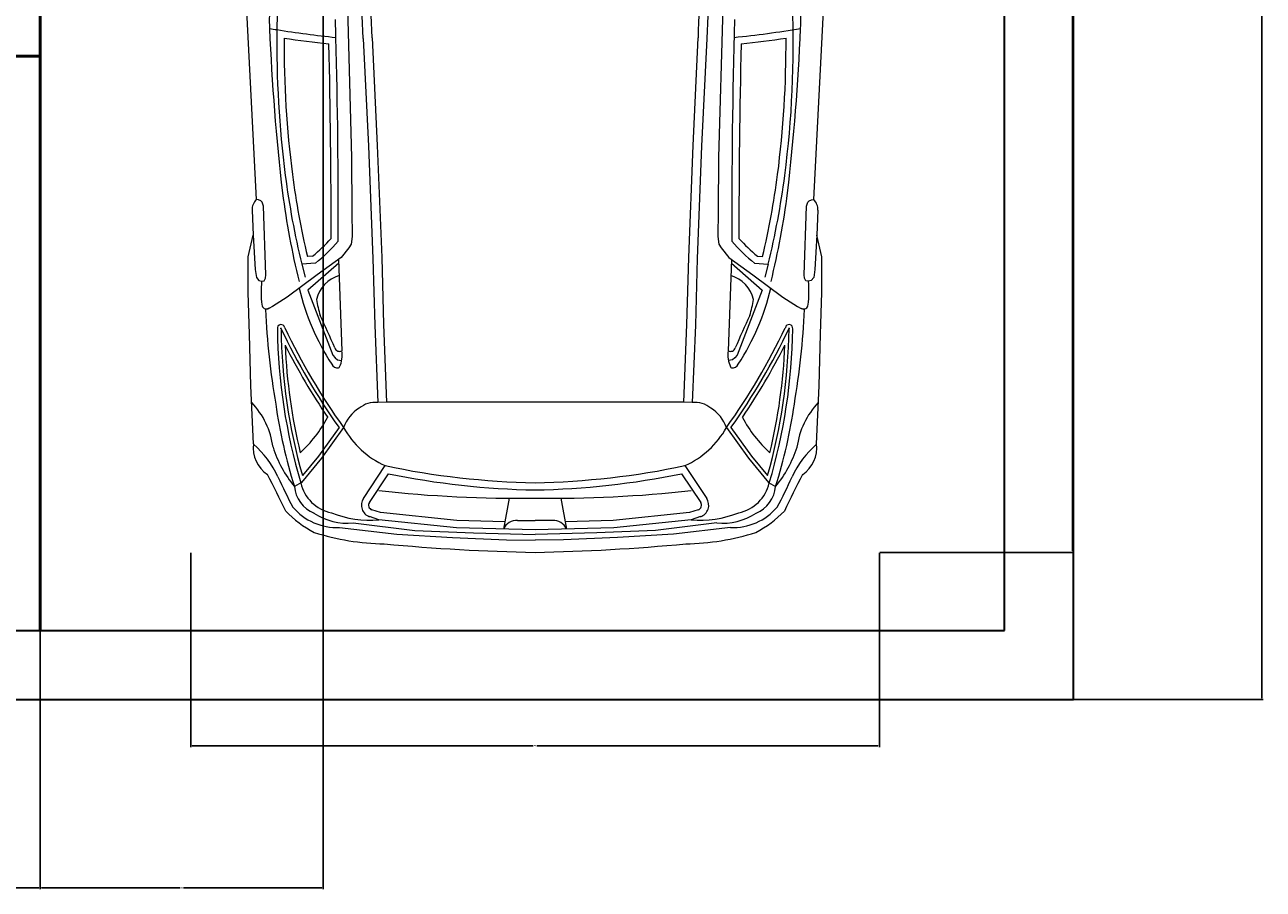
# Model space of a CAD drawing. Units: inches. Extents: x 8049 to 8459, y 820 to 1350.
# Tile 20 of 25: x 8297 to 8459, y 820 to 933. Entities that reach past the tile are written whole.
import ezdxf

# ---------------------------------------------------------------- set-up
doc = ezdxf.new("R2010")
doc.units = ezdxf.units.IN
doc.header["$MEASUREMENT"] = 0
for name, color, linetype, lineweight in [('A-ANNO-DIMS', 2, 'Continuous', 18), ('A-WALL', 7, 'Continuous', 50), ('C-PKNG-VEH', 8, 'Continuous', 13), ('C-SITE-WALL', 7, 'Continuous', 35)]:
    doc.layers.add(name, color=color, linetype=linetype, lineweight=lineweight)
doc.styles.get("Standard").update_dxf_attribs({"font": 'arial.ttf'})
doc.dimstyles.get("Standard").update_dxf_attribs({"dimtxt": 0.18, "dimasz": 0.18, "dimexe": 0.18, "dimexo": 0.0625, "dimgap": 0.09, "dimtad": 0, "dimtih": 1, "dimtoh": 1, "dimdec": 4, "dimzin": 0, "dimdsep": 46, "dimtxsty": 'Standard', "dimcen": 0.09, "dimadec": 0, "dimazin": 0, "dimtfac": 1, "dimtdec": 4, "dimtofl": 0, "dimtmove": 0, "dimatfit": 3, "dimfxl": 1, "dimtolj": 1, "dimtzin": 0, "dimarcsym": 0})

# ---------------------------------------------------------------- blocks, each defined once
blk = doc.blocks.new('A$C27D64469')
for p, q in [((-0.5059, -2.4594), (-0.4945, -2.8747)), ((0.5331, -2.4594), (0.5216, -2.8747)), ((-0.4622, -2.5454), (-0.4477, -2.8433)), ((-0.4375, -2.5434), (-0.423, -2.8413)), ((0.4646, -2.5434), (0.4501, -2.8413)), ((0.4894, -2.5454), (0.4748, -2.8433)), ((-0.4477, -2.8433), (-0.4357, -3.1539)), ((-0.423, -2.8413), (-0.4109, -3.152)), ((0.4501, -2.8413), (0.4381, -3.152)), ((0.4748, -2.8433), (0.4628, -3.1539)), ((-0.4945, -2.8747), (-0.4935, -3.0236)), ((0.5216, -2.8747), (0.5207, -3.0236)), ((-0.7516, -2.9924), (-0.758, -2.9914)), ((-0.7456, -2.9946), (-0.7516, -2.9924)), ((-0.7413, -2.9989), (-0.7456, -2.9946)), ((-0.738, -3.0096), (-0.7413, -2.9989)), ((-0.7319, -3.1994), (-0.738, -3.0096)), ((0.759, -3.1994), (0.7651, -3.0096)), ((0.7651, -3.0096), (0.7684, -2.9989)), ((0.7684, -2.9989), (0.7727, -2.9946)), ((0.7727, -2.9946), (0.7788, -2.9924)), ((0.7788, -2.9924), (0.7852, -2.9914)), ((-0.7694, -3.0205), (-0.7665, -3.0897)), ((-0.4935, -3.0236), (-0.4926, -3.0933)), ((0.5207, -3.0236), (0.5197, -3.0933)), ((0.7965, -3.0205), (0.7936, -3.0897)), ((-0.7802, -3.1498), (-0.7665, -3.0897)), ((-0.7665, -3.0897), (-0.761, -3.1849)), ((-0.4954, -3.115), (-0.502, -3.1244)), ((-0.4926, -3.0933), (-0.4954, -3.115)), ((0.5197, -3.0933), (0.5226, -3.115)), ((0.5226, -3.115), (0.5292, -3.1244)), ((0.7936, -3.0897), (0.7882, -3.1849)), ((0.8074, -3.1498), (0.7936, -3.0897)), ((-0.7802, -3.248), (-0.7802, -3.1498)), ((-0.6019, -3.1478), (-0.6165, -3.1489)), ((-0.5227, -3.1517), (-0.5896, -3.1998)), ((-0.502, -3.1244), (-0.5227, -3.1517)), ((-0.4109, -3.152), (-0.4055, -3.3366)), ((0.4381, -3.152), (0.4327, -3.3366)), ((0.5292, -3.1244), (0.5499, -3.1517)), ((0.5499, -3.1517), (0.6167, -3.1998)), ((0.6291, -3.1478), (0.6437, -3.1489)), ((0.8074, -3.248), (0.8074, -3.1498)), ((-0.761, -3.1849), (-0.7577, -3.207)), ((-0.594, -3.1673), (-0.632, -3.1701)), ((-0.632, -3.1701), (-0.6229, -3.206)), ((-0.5298, -3.1676), (-0.615, -3.2421)), ((-0.5302, -3.1571), (-0.5208, -3.4098)), ((-0.4357, -3.1539), (-0.4303, -3.3385)), ((0.4628, -3.1539), (0.4574, -3.3385)), ((0.5573, -3.1571), (0.548, -3.4098)), ((0.557, -3.1676), (0.6422, -3.2421)), ((0.6212, -3.1673), (0.6592, -3.1701)), ((0.6592, -3.1701), (0.65, -3.206)), ((0.7882, -3.1849), (0.7849, -3.207)), ((-0.7577, -3.207), (-0.7506, -3.2153)), ((-0.7506, -3.2153), (-0.743, -3.2171)), ((-0.743, -3.2171), (-0.7359, -3.2158)), ((-0.7359, -3.2158), (-0.7324, -3.2087)), ((-0.7324, -3.2087), (-0.7319, -3.1994)), ((-0.5896, -3.1998), (-0.6725, -3.261)), ((0.6167, -3.1998), (0.6996, -3.261)), ((0.7595, -3.2087), (0.759, -3.1994)), ((0.7631, -3.2158), (0.7595, -3.2087)), ((0.7702, -3.2171), (0.7631, -3.2158)), ((0.7778, -3.2153), (0.7702, -3.2171)), ((0.7849, -3.207), (0.7778, -3.2153)), ((-0.777, -3.3641), (-0.7802, -3.248)), ((-0.615, -3.2421), (-0.5463, -3.4221)), ((0.6422, -3.2421), (0.5734, -3.4221)), ((0.8042, -3.3641), (0.8074, -3.248)), ((-0.713, -3.2874), (-0.7233, -3.2925)), ((-0.6725, -3.261), (-0.713, -3.2874)), ((0.6996, -3.261), (0.7401, -3.2874)), ((0.7401, -3.2874), (0.7505, -3.2925)), ((-0.7224, -3.2921), (-0.7327, -3.2955)), ((0.7495, -3.2921), (0.7599, -3.2955)), ((-0.4303, -3.3385), (-0.4218, -3.5529)), ((-0.4055, -3.3366), (-0.3971, -3.5519)), ((0.4327, -3.3366), (0.4242, -3.5519)), ((0.4574, -3.3385), (0.449, -3.5529)), ((-0.7728, -3.5066), (-0.777, -3.3641)), ((0.8, -3.5066), (0.8042, -3.3641)), ((-0.5463, -3.4221), (-0.5397, -3.4296)), ((0.5734, -3.4221), (0.5668, -3.4296)), ((-0.5397, -3.4296), (-0.5331, -3.4343)), ((-0.5331, -3.4343), (-0.5217, -3.4366)), ((0.5602, -3.4343), (0.5488, -3.4366)), ((0.5668, -3.4296), (0.5602, -3.4343)), ((-0.7654, -3.667), (-0.7728, -3.5066)), ((0.7926, -3.667), (0.8, -3.5066)), ((-0.3971, -3.5519), (-0.4218, -3.5529)), ((0.0136, -3.5519), (-0.3971, -3.5519)), ((0.4242, -3.5519), (0.0136, -3.5519)), ((0.449, -3.5529), (0.4242, -3.5519)), ((-0.5287, -3.6221), (-0.5854, -3.701)), ((-0.5163, -3.6221), (-0.5774, -3.7071)), ((0.5435, -3.6221), (0.6046, -3.7071)), ((0.5559, -3.6221), (0.6126, -3.701)), ((-0.5854, -3.701), (-0.6302, -3.755)), ((0.6126, -3.701), (0.6574, -3.755)), ((-0.5774, -3.7071), (-0.6331, -3.7742)), ((-0.4616, -3.818), (-0.4014, -3.7275)), ((0.4285, -3.7275), (0.4887, -3.818)), ((0.6046, -3.7071), (0.6602, -3.7742)), ((-0.4449, -3.8291), (-0.3922, -3.7498)), ((0.4193, -3.7498), (0.4721, -3.8291)), ((-0.6331, -3.7742), (-0.6525, -3.7849)), ((0.6602, -3.7742), (0.6796, -3.7849)), ((-0.0581, -3.8176), (-0.0735, -3.9028)), ((0.0853, -3.8176), (0.1006, -3.9028)), ((-0.4185, -3.8772), (-0.4442, -3.8686)), ((-0.4142, -3.8575), (-0.4379, -3.8496)), ((-0.2029, -3.8795), (-0.4142, -3.8575)), ((0.4414, -3.8575), (0.2301, -3.8795)), ((0.465, -3.8496), (0.4414, -3.8575)), ((0.4713, -3.8686), (0.4456, -3.8772)), ((-0.5278, -3.8988), (-0.3693, -3.9174)), ((-0.4897, -3.8861), (-0.3195, -3.9066)), ((-0.2042, -3.8994), (-0.4185, -3.8772)), ((-0.3195, -3.9066), (-0.1571, -3.9135)), ((0.0136, -3.905), (-0.2042, -3.8994)), ((-0.0699, -3.8829), (-0.2029, -3.8795)), ((-0.0347, -3.8792), (0.0136, -3.8792)), ((0.0618, -3.8792), (0.0136, -3.8792)), ((0.2314, -3.8994), (0.0136, -3.905)), ((0.2301, -3.8795), (0.097, -3.8829)), ((0.3466, -3.9066), (0.1842, -3.9135)), ((0.4456, -3.8772), (0.2314, -3.8994)), ((0.5168, -3.8861), (0.3466, -3.9066)), ((0.5549, -3.8988), (0.3965, -3.9174)), ((-0.3693, -3.9174), (-0.2148, -3.9262)), ((-0.2148, -3.9262), (-0.0652, -3.933)), ((-0.1571, -3.9135), (0.0136, -3.9184)), ((-0.0652, -3.933), (0.0136, -3.934)), ((0.1842, -3.9135), (0.0136, -3.9184)), ((0.0923, -3.933), (0.0136, -3.934)), ((0.242, -3.9262), (0.0923, -3.933)), ((0.3965, -3.9174), (0.242, -3.9262))]:
    blk.add_line(p, q)
for centre, radius, start, end in [((-11.1621, -2.9794), 10.7086, 2.32274, 4.10377), ((-11.1373, -2.9775), 10.7086, 2.32274, 4.10377), ((11.1645, -2.9775), 10.7086, 175.89623, 177.67726), ((11.1892, -2.9794), 10.7086, 175.89623, 177.67726), ((145.5619, 4.7984), 146.5271, 182.82189, 183.047472), ((-145.5348, 4.7984), 146.5271, 356.952528, 357.17811), ((-0.4463, -2.4963), 0.2758, 169.4971, 184.519), ((2.1845, -2.5566), 2.8858, 177.9428, 179.2929), ((-2.1573, -2.5566), 2.8858, 352.6735, 2.0572), ((0.4735, -2.4963), 0.2758, 355.481, 10.5029), ((-21.144, -3.0635), 20.6131, 1.44842, 1.58522), ((21.1711, -3.0635), 20.6131, 178.41478, 180.12035), ((-0.2547, 0.2402), 2.7971, 260.3968, 260.8181), ((5.4584, -2.2589), 6.1852, 182.40058, 186.62429), ((2.1845, -2.5566), 2.8858, 179.2929, 187.3265), ((-0.2547, 0.2402), 2.7971, 260.8181, 264.1988), ((0.2819, 0.2402), 2.7971, 275.8012, 279.6032), ((-5.4313, -2.2589), 6.1852, 353.37571, 357.59942), ((-0.2547, 0.2402), 2.8171, 261.2916, 263.8402), ((2.1845, -2.5566), 2.8658, 179.7551, 187.3262), ((-21.144, -3.0635), 20.5931, 359.90118, 1.39956), ((-21.144, -3.0635), 20.6131, 359.87965, 1.44842), ((21.1711, -3.0635), 20.5931, 178.60044, 180.09882), ((0.2819, 0.2402), 2.8171, 276.1598, 278.7084), ((-2.1573, -2.5566), 2.8658, 352.6738, 0.2449), ((1.5917, -2.6291), 2.2886, 187.4191, 193.6744), ((1.5917, -2.6291), 2.2686, 187.4195, 193.2465), ((-1.5646, -2.6291), 2.2686, 346.7535, 352.5805), ((-1.5646, -2.6291), 2.2886, 346.3256, 352.5809), ((1.584, -2.6769), 2.2886, 187.4191, 193.6744), ((-1.5568, -2.6769), 2.2886, 346.3256, 352.5809), ((-0.7323, -3.0182), 0.0371, 133.8458, 183.4773), ((0.7594, -3.0182), 0.0371, 356.5227, 46.1542), ((-0.9762, -2.7051), 0.5797, 310.2112, 317.1922), ((-0.9762, -2.7051), 0.5997, 309.5861, 317.9444), ((1.0033, -2.7051), 0.5997, 222.0556, 230.4139), ((1.0033, -2.7051), 0.5797, 222.8078, 229.7888), ((-0.4258, -3.2462), 0.3189, 174.7532, 186.4501), ((-0.5023, -3.2896), 0.0919, 106.6274, 166.1462), ((0.5294, -3.2896), 0.0919, 13.8538, 73.3726), ((0.4529, -3.2462), 0.3189, 353.5499, 5.2468), ((-0.0025, -3.0882), 0.6536, 193.0984, 213.2489), ((0.0296, -3.0882), 0.6536, 326.7511, 346.9016), ((-0.7293, -3.2805), 0.0135, 186.4501, 296.5725), ((-0.2573, -3.2127), 0.3386, 189.3185, 197.018), ((0.2844, -3.2127), 0.3386, 342.982, 350.6815), ((0.7565, -3.2805), 0.0135, 243.4275, 353.5499), ((1.5487, -3.1796), 2.2844, 182.9075, 189.515), ((-6.7047, -6.1366), 6.7437, 23.9284, 24.763), ((6.7318, -6.1366), 6.7437, 155.237, 156.0716), ((-1.5216, -3.1796), 2.2844, 350.485, 357.0925), ((-0.6895, -3.3475), 0.0103, 9.7306, 189.7306), ((0.8768, -3.3275), 1.5766, 180.7904, 196.499), ((-0.6895, -3.3475), 0.000207, 234.3096, 189.7306), ((-0.6997, -3.3492), 0.0101, 0.7904, 9.7306), ((0.9825, -2.5519), 1.8518, 205.4494, 215.3046), ((0.8768, -3.3275), 1.5665, 180.7904, 195.8378), ((0.9825, -2.5519), 1.8417, 205.5332, 215.5287), ((-0.9554, -2.5519), 1.8417, 324.4713, 334.4668), ((-0.9554, -2.5519), 1.8518, 324.6954, 334.5506), ((-0.8496, -3.3275), 1.5665, 344.1622, 359.2096), ((-0.8496, -3.3275), 1.5766, 343.501, 359.2096), ((0.7166, -3.3475), 0.0103, 350.2694, 170.2694), ((0.7166, -3.3475), 0.000207, 350.2694, 305.6904), ((0.7268, -3.3492), 0.0101, 170.2694, 179.2096), ((0.8768, -3.3275), 1.5564, 182.4426, 193.5531), ((0.9825, -2.5519), 1.8619, 206.8832, 214.0379), ((-0.9554, -2.5519), 1.8619, 325.9621, 333.1168), ((-0.8496, -3.3275), 1.5564, 346.4469, 357.5574), ((-0.5273, -3.3975), 0.0139, 196.0998, 297.49), ((-0.5991, -3.4208), 0.079, 335.0797, 7.9846), ((0.6263, -3.4208), 0.079, 172.0154, 204.9203), ((0.5544, -3.3975), 0.0139, 242.51, 343.9002), ((-0.5332, -3.4402), 0.0172, 201.6995, 279.6425), ((-0.5326, -3.4521), 0.00559, 294.9923, 338.6694), ((0.5598, -3.4521), 0.00559, 201.3306, 245.0077), ((0.5603, -3.4402), 0.0172, 260.3575, 338.3005), ((-0.931, -3.7054), 0.2213, 7.498, 43.5729), ((0.6722, -3.364), 1.3899, 187.9913, 197.6257), ((-0.4293, -3.6198), 0.0673, 83.5915, 130.4352), ((0.4565, -3.6198), 0.0673, 49.5648, 96.4085), ((-0.645, -3.364), 1.3899, 342.3743, 352.0087), ((0.9581, -3.7054), 0.2213, 136.4271, 172.502), ((-0.9014, -3.4088), 0.388, 313.0938, 331.4872), ((-0.421, -3.6549), 0.1008, 121.0416, 161.032), ((0.4482, -3.6549), 0.1008, 18.968, 58.9584), ((0.9285, -3.4088), 0.388, 208.5128, 226.9062), ((-0.3005, -3.502), 0.247, 209.0915, 245.8956), ((0.3276, -3.502), 0.247, 294.1044, 330.9085), ((-0.6785, -3.679), 0.0877, 172.132, 236.2396), ((0.7057, -3.679), 0.0877, 303.7604, 7.868), ((-0.9429, -3.8711), 0.2695, 24.6265, 48.8595), ((-0.3962, -3.5747), 0.3315, 197.8909, 219.3552), ((0.4233, -3.5747), 0.3315, 320.6448, 342.1091), ((0.97, -3.8711), 0.2695, 131.1405, 155.3735), ((0.0567, -1.5526), 2.2226, 258.1061, 268.8881), ((-0.0296, -1.5526), 2.2226, 271.1119, 281.8939), ((-3.375, -5.1387), 2.9889, 25.4724, 27.6425), ((0.5567, -3.1915), 1.3769, 204.3314, 208.2014), ((0.0567, -1.5526), 2.2426, 258.453, 268.898), ((-0.0296, -1.5526), 2.2426, 271.102, 281.547), ((-0.5295, -3.1915), 1.3769, 331.7986, 335.6686), ((3.4021, -5.1387), 2.9889, 152.3575, 154.5276), ((-0.566, -3.7782), 0.0867, 184.4324, 248.21), ((-0.528, -3.7506), 0.1097, 192.9436, 258.3207), ((-0.0346, -0.3333), 3.4843, 263.6749, 270.7924), ((0.0618, -0.3333), 3.4843, 269.2076, 276.3251), ((0.5551, -3.7506), 0.1097, 281.6793, 347.0564), ((0.5932, -3.7782), 0.0867, 291.79, 355.5676), ((-0.4335, -3.8367), 0.0337, 146.3764, 251.5583), ((-0.4335, -3.8367), 0.0137, 146.3764, 251.5583), ((0.4607, -3.8367), 0.0137, 288.4417, 33.6236), ((0.4607, -3.8367), 0.0337, 288.4417, 33.6236), ((-0.4633, -3.6496), 0.2949, 223.6549, 242.8613), ((-0.5341, -3.738), 0.1609, 220.3568, 272.2613), ((-0.5047, -3.7168), 0.17, 236.6049, 275.0704), ((-0.4436, -3.5867), 0.2916, 248.5479, 274.9353), ((0.4707, -3.5867), 0.2916, 265.0647, 291.4521), ((0.5318, -3.7168), 0.17, 264.9296, 303.3951), ((0.5613, -3.738), 0.1609, 267.7387, 319.6432), ((0.4904, -3.6496), 0.2949, 297.1387, 316.3451), ((-0.0379, -3.9176), 0.0386, 85.1824, 157.357), ((0.065, -3.9176), 0.0386, 22.643, 94.8176), ((-0.3932, -3.2709), 0.673, 252.2974, 269.1096), ((0.4203, -3.2709), 0.673, 270.8904, 287.7026), ((0.1171, 1.5736), 5.542, 264.6089, 268.93), ((-0.0899, 1.5736), 5.542, 271.07, 275.3911)]:
    blk.add_arc(centre, radius, start, end)
blk = doc.blocks.new('*D46')
at = {"layer": 'A-ANNO-DIMS', "color": 0, "lineweight": -2, "transparency": 16777216}
for p, q in [((8409.11, 1032.41), (8434.48, 1032.41)), ((8434.3, 1032.23), (8434.3, 948.43)), ((8434.3, 864.26), (8434.3, 948.06)), ((8409.11, 864.08), (8434.48, 864.08))]:
    blk.add_line(p, q, dxfattribs=at)
at = {"layer": 'A-ANNO-DIMS', "color": 0, "transparency": 16777216}
for points in [[(8434.27, 1032.23), (8434.33, 1032.23), (8434.3, 1032.41)], [(8434.27, 864.26), (8434.33, 864.26), (8434.3, 864.08)]]:
    blk.add_solid(points, dxfattribs=at)
at = {"layer": 'Defpoints', "color": 0, "transparency": 16777216}
for p in [(8409.05, 1032.41), (8434.3, 1032.41), (8409.05, 864.08)]:
    blk.add_point(p, dxfattribs=at)
at = {"layer": 'A-ANNO-DIMS', "color": 0, "transparency": 16777216, "insert": (8434.3, 948.24), "char_height": 0.18, "attachment_point": 5}
blk.add_mtext('\\A1;CAR 168', dxfattribs=at)
blk = doc.blocks.new('*D47')
at = {"layer": 'A-ANNO-DIMS', "color": 0, "lineweight": -2, "transparency": 16777216}
for p, q in [((8319.08, 864.02), (8319.08, 838.65)), ((8409.05, 864.02), (8409.05, 838.65)), ((8319.26, 838.83), (8363.84, 838.83)), ((8408.87, 838.83), (8364.28, 838.83))]:
    blk.add_line(p, q, dxfattribs=at)
at = {"layer": 'A-ANNO-DIMS', "color": 0, "transparency": 16777216}
for points in [[(8319.26, 838.86), (8319.26, 838.8), (8319.08, 838.83)], [(8408.87, 838.86), (8408.87, 838.8), (8409.05, 838.83)]]:
    blk.add_solid(points, dxfattribs=at)
at = {"layer": 'Defpoints', "color": 0, "transparency": 16777216}
for p in [(8319.08, 864.08), (8409.05, 864.08), (8409.05, 838.83)]:
    blk.add_point(p, dxfattribs=at)
at = {"layer": 'A-ANNO-DIMS', "color": 0, "transparency": 16777216, "insert": (8364.06, 838.83), "char_height": 0.18, "attachment_point": 5}
blk.add_mtext('\\A1;90', dxfattribs=at)
blk = doc.blocks.new('*D49')
at = {"layer": 'A-ANNO-DIMS', "color": 0, "lineweight": -2, "transparency": 16777216}
for p, q in [((8434.46, 1324.87), (8459.18, 1324.87)), ((8459, 1324.69), (8459, 1085.05)), ((8459, 845.05), (8459, 1084.69)), ((8434.46, 844.87), (8459.18, 844.87))]:
    blk.add_line(p, q, dxfattribs=at)
at = {"layer": 'A-ANNO-DIMS', "color": 0, "transparency": 16777216}
for points in [[(8458.97, 1324.69), (8459.03, 1324.69), (8459, 1324.87)], [(8458.97, 845.05), (8459.03, 845.05), (8459, 844.87)]]:
    blk.add_solid(points, dxfattribs=at)
at = {"layer": 'Defpoints', "color": 0, "transparency": 16777216}
for p in [(8434.4, 1324.87), (8459, 1324.87), (8434.4, 844.87)]:
    blk.add_point(p, dxfattribs=at)
at = {"layer": 'A-ANNO-DIMS', "color": 0, "transparency": 16777216, "insert": (8459, 1084.87), "char_height": 0.18, "attachment_point": 5}
blk.add_mtext('\\A1;480', dxfattribs=at)
blk = doc.blocks.new('*D66')
at = {"layer": 'A-ANNO-DIMS', "color": 0, "lineweight": -2, "transparency": 16777216}
for p, q in [((8336.4, 1267.81), (8336.4, 820.09)), ((8299.4, 1258.81), (8299.4, 820.09)), ((8299.58, 820.27), (8317.68, 820.27)), ((8336.22, 820.27), (8318.12, 820.27))]:
    blk.add_line(p, q, dxfattribs=at)
at = {"layer": 'A-ANNO-DIMS', "color": 0, "transparency": 16777216}
for points in [[(8299.58, 820.3), (8299.58, 820.24), (8299.4, 820.27)], [(8336.22, 820.3), (8336.22, 820.24), (8336.4, 820.27)]]:
    blk.add_solid(points, dxfattribs=at)
at = {"layer": 'Defpoints', "color": 0, "transparency": 16777216}
for p in [(8336.4, 1267.87), (8299.4, 1258.87), (8299.4, 820.27)]:
    blk.add_point(p, dxfattribs=at)
at = {"layer": 'A-ANNO-DIMS', "color": 0, "transparency": 16777216, "insert": (8317.9, 820.27), "char_height": 0.18, "attachment_point": 5}
blk.add_mtext('\\A1;37', dxfattribs=at)
blk = doc.blocks.new('*D76')
at = {"layer": 'A-ANNO-DIMS', "color": 0, "lineweight": -2, "transparency": 16777216}
for p, q in [((8083.4, 1054.81), (8083.4, 820.09)), ((8299.4, 1054.81), (8299.4, 820.09)), ((8083.58, 820.27), (8191.11, 820.27)), ((8299.22, 820.27), (8191.69, 820.27))]:
    blk.add_line(p, q, dxfattribs=at)
at = {"layer": 'A-ANNO-DIMS', "color": 0, "transparency": 16777216}
for points in [[(8083.58, 820.3), (8083.58, 820.24), (8083.4, 820.27)], [(8299.22, 820.3), (8299.22, 820.24), (8299.4, 820.27)]]:
    blk.add_solid(points, dxfattribs=at)
at = {"layer": 'Defpoints', "color": 0, "transparency": 16777216}
for p in [(8083.4, 1054.87), (8299.4, 1054.87), (8299.4, 820.27)]:
    blk.add_point(p, dxfattribs=at)
at = {"layer": 'A-ANNO-DIMS', "color": 0, "transparency": 16777216, "insert": (8191.4, 820.27), "char_height": 0.18, "attachment_point": 5}
blk.add_mtext('\\A1;216', dxfattribs=at)

msp = doc.modelspace()

# ---------------------------------------------------------------- linework, layer by layer
at = {"layer": 'A-WALL'}
for p, q in [((8299.3974, 853.8706), (8299.3974, 1045.8706)), ((8299.3974, 928.8706), (8221.3974, 928.8706))]:
    msp.add_line(p, q, dxfattribs=at)
at = {"layer": 'C-SITE-WALL'}
for p, q in [((8434.3974, 844.8706), (8434.3974, 1324.8706)), ((8425.3974, 853.8706), (8425.3974, 1315.8706)), ((8267.8765, 853.8706), (8425.3974, 853.8706)), ((8267.8974, 844.8706), (8434.3974, 844.8706))]:
    msp.add_line(p, q, dxfattribs=at)

# ---------------------------------------------------------------- block references
at = {"layer": 'C-PKNG-VEH', "xscale": 47.19862401584114, "yscale": 47.19862401584114, "zscale": 47.19862401584114}
msp.add_blockref('A$C27D64469', (8363.4216, 1051.3375), dxfattribs=at)

# ---------------------------------------------------------------- dimensions: what is measured, and where the dimension line sits
at = {"layer": 'A-ANNO-DIMS'}
dim = msp.add_linear_dim(base=(8458.9974, 1324.8706), p1=(8434.3974, 844.8706), p2=(8434.3974, 1324.8706), angle=90, dimstyle='Standard', override={"dimdec": 0, "dimlfac": 1, "dimrnd": 0, "dimzin": 0, "dimdsep": 46, "dimlunit": 2}, dxfattribs=at)
dim.commit()
dim.dimension.update_dxf_attribs({"geometry": '*D49', "text_midpoint": (8458.9974, 1084.8706)})
for base, p1, p2, picture, middle in [((8299.3974, 820.2706), (8336.3974, 1267.8706), (8299.3974, 1258.8706), '*D66', (8317.8974, 820.2706)), ((8299.3974, 820.2706), (8083.3974, 1054.8706), (8299.3974, 1054.8706), '*D76', (8191.3974, 820.2706)), ((8409.0493, 838.8317), (8319.075, 864.0808), (8409.0493, 864.0808), '*D47', (8364.0621, 838.8317))]:
    dim = msp.add_linear_dim(base=base, p1=p1, p2=p2, dimstyle='Standard', override={"dimdec": 0, "dimlfac": 1, "dimrnd": 0, "dimzin": 0, "dimdsep": 46, "dimlunit": 2}, dxfattribs=at)
    dim.commit()
    dim.dimension.update_dxf_attribs({"geometry": picture, "text_midpoint": middle})
dim = msp.add_linear_dim(base=(8434.2984, 1032.4086), p1=(8409.0493, 864.0808), p2=(8409.0493, 1032.4086), angle=90, text='CAR <>', dimstyle='Standard', override={"dimdec": 0, "dimlfac": 1, "dimrnd": 0, "dimzin": 0, "dimdsep": 46, "dimlunit": 2}, dxfattribs=at)
dim.commit()
dim.dimension.update_dxf_attribs({"geometry": '*D46', "text_midpoint": (8434.2984, 948.2447)})

doc.saveas('drawing.dxf')
